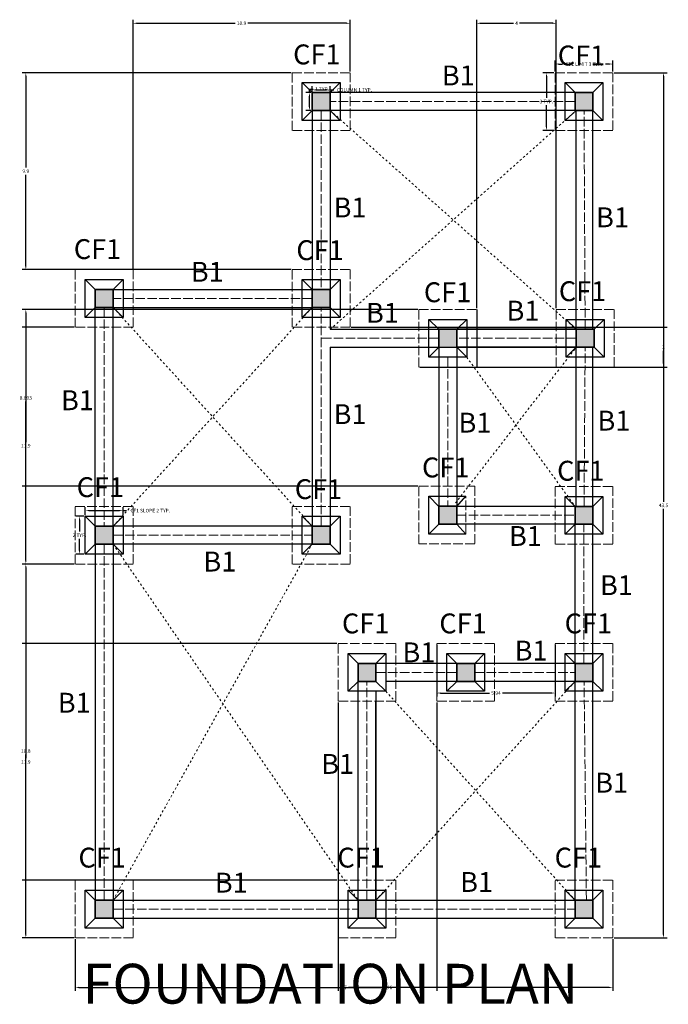
# Model space of a CAD drawing. Units: inches. Extents: x -193.8 to -127.9, y -122.4 to -72.3.
# Tile 2 of 2: x -160.4 to -127.9, y -121.8 to -72.3. Entities that reach past the tile are written whole.
import ezdxf

# ---------------------------------------------------------------- set-up
doc = ezdxf.new("R2010")
doc.units = ezdxf.units.IN
doc.header["$LTSCALE"] = 0.2
doc.header["$MEASUREMENT"] = 0
doc.linetypes.add('ACAD_ISO02W100', pattern=[15, 12, -3])
doc.linetypes.add('ACAD_ISO07W100', pattern=[3, 0, -3])
for name, color, linetype, lineweight in [('A-ANNO-DIMS', 2, 'Continuous', 18), ('S-ANNO-TEXT', 7, 'Continuous', 18), ('S-ANNO-TITL', 2, 'Continuous', 35), ('S-BEAM', 7, 'Continuous', 30), ('S-BEAM-CNTR', 8, 'ACAD_ISO02W100', 13), ('S-COLS', 7, 'Continuous', 35), ('S-COLS-PATT', 252, 'Continuous', 13), ('S-FNDN', 3, 'Continuous', 25), ('S-FNDN-DIAG', 8, 'ACAD_ISO07W100', 13), ('S-FNDN-HIDN', 3, 'ACAD_ISO02W100', 18)]:
    doc.layers.add(name, color=color, linetype=linetype, lineweight=lineweight)
doc.styles.get("Standard").update_dxf_attribs({"font": 'arial.ttf'})
doc.dimstyles.get("Standard").update_dxf_attribs({"dimtxt": 0.18, "dimasz": 0.18, "dimexe": 0.18, "dimexo": 0.0625, "dimgap": 0.09, "dimtad": 0, "dimtih": 1, "dimtoh": 1, "dimdec": 1, "dimzin": 0, "dimdsep": 46, "dimlunit": 4, "dimtxsty": 'Standard', "dimcen": 0.09, "dimadec": 0, "dimazin": 0, "dimtfac": 1, "dimtdec": 1, "dimtofl": 0, "dimtmove": 0, "dimatfit": 3, "dimfxl": 1, "dimtolj": 1, "dimtzin": 0, "dimarcsym": 0})

# ---------------------------------------------------------------- blocks, each defined once
blk = doc.blocks.new('FOOTING-CF1-SLOPED')
for p, q in [((0, 0), (0, 1.9)), ((0, 1.9), (1.9, 1.9)), ((1.9, 1.9), (1.9, 0)), ((1.9, 0), (0, 0))]:
    blk.add_line(p, q)
at = {"ltscale": 0.2}
for p, q in [((0, 1.9), (0.5, 1.4)), ((1.4, 1.4), (1.9, 1.9)), ((0, 0), (0.5, 0.5)), ((1.4, 0.5), (1.9, 0))]:
    blk.add_line(p, q, dxfattribs=at)
blk = doc.blocks.new('FOOTING-CF1-LIMIT')
at = {"ltscale": 0.2}
for p, q in [((0, 2.9), (2.9, 2.9)), ((0, 0), (0, 2.9)), ((2.9, 2.9), (2.9, 0)), ((2.9, 0), (0, 0))]:
    blk.add_line(p, q, dxfattribs=at)
blk = doc.blocks.new('COLUMN-SQUARE-PLAN')
for p, q in [((0, 0.9), (0.9, 0.9)), ((0, 0), (0, 0.9)), ((0.9, 0.9), (0.9, 0)), ((0.9, 0), (0, 0))]:
    blk.add_line(p, q)
blk = doc.blocks.new('*D19')
at = {"layer": 'A-ANNO-DIMS', "color": 0, "lineweight": -2, "ltscale": 0.2, "transparency": 16777216}
for p, q in [((-157.135, -97.158), (-157.135, -96.755)), ((-156.955, -96.935), (-155.415, -96.935)), ((-155.235, -97.158), (-155.235, -96.755)), ((-155.235, -96.935), (-155.055, -96.935))]:
    blk.add_line(p, q, dxfattribs=at)
at = {"layer": 'A-ANNO-DIMS', "color": 0, "ltscale": 0.2, "transparency": 16777216}
for points in [[(-156.955, -96.905), (-156.955, -96.965), (-157.135, -96.935)], [(-155.415, -96.905), (-155.415, -96.965), (-155.235, -96.935)]]:
    blk.add_solid(points, dxfattribs=at)
at = {"layer": 'Defpoints', "color": 0, "ltscale": 0.2, "transparency": 16777216}
for p in [(-155.235, -96.935), (-157.135, -97.22), (-155.235, -97.22)]:
    blk.add_point(p, dxfattribs=at)
at = {"layer": 'A-ANNO-DIMS', "color": 0, "ltscale": 0.2, "transparency": 16777216, "insert": (-153.871, -96.935), "char_height": 0.18, "attachment_point": 5}
blk.add_mtext('\\A1;CF1 SLOPE 2 TYP.', dxfattribs=at)
blk = doc.blocks.new('*D20')
at = {"layer": 'A-ANNO-DIMS', "color": 0, "lineweight": -2, "ltscale": 0.2, "transparency": 16777216}
for p, q in [((-157.198, -97.22), (-157.6, -97.22)), ((-157.42, -97.4), (-157.42, -97.99)), ((-157.42, -98.94), (-157.42, -98.35)), ((-157.198, -99.12), (-157.6, -99.12))]:
    blk.add_line(p, q, dxfattribs=at)
at = {"layer": 'A-ANNO-DIMS', "color": 0, "ltscale": 0.2, "transparency": 16777216}
for points in [[(-157.45, -97.4), (-157.39, -97.4), (-157.42, -97.22)], [(-157.45, -98.94), (-157.39, -98.94), (-157.42, -99.12)]]:
    blk.add_solid(points, dxfattribs=at)
at = {"layer": 'Defpoints', "color": 0, "ltscale": 0.2, "transparency": 16777216}
for p in [(-157.42, -97.22), (-157.135, -97.22), (-157.135, -99.12)]:
    blk.add_point(p, dxfattribs=at)
at = {"layer": 'A-ANNO-DIMS', "color": 0, "ltscale": 0.2, "transparency": 16777216, "insert": (-157.42, -98.17), "char_height": 0.18, "attachment_point": 5}
blk.add_mtext('\\A1;2 TYP.', dxfattribs=at)
blk = doc.blocks.new('*D21')
at = {"layer": 'A-ANNO-DIMS', "color": 0, "lineweight": -2, "ltscale": 0.2, "transparency": 16777216}
for p, q in [((-133.535, -74.858), (-133.535, -74.305)), ((-133.355, -74.485), (-133.171, -74.485)), ((-130.815, -74.485), (-130.999, -74.485)), ((-130.635, -74.858), (-130.635, -74.305))]:
    blk.add_line(p, q, dxfattribs=at)
at = {"layer": 'A-ANNO-DIMS', "color": 0, "ltscale": 0.2, "transparency": 16777216}
for points in [[(-133.355, -74.455), (-133.355, -74.515), (-133.535, -74.485)], [(-130.815, -74.455), (-130.815, -74.515), (-130.635, -74.485)]]:
    blk.add_solid(points, dxfattribs=at)
at = {"layer": 'Defpoints', "color": 0, "ltscale": 0.2, "transparency": 16777216}
for p in [(-133.535, -74.485), (-133.535, -74.92), (-130.635, -74.92)]:
    blk.add_point(p, dxfattribs=at)
at = {"layer": 'A-ANNO-DIMS', "color": 0, "ltscale": 0.2, "transparency": 16777216, "insert": (-132.085, -74.485), "char_height": 0.18, "attachment_point": 5}
blk.add_mtext('\\A1;CF1 LIMIT 3 TYP.', dxfattribs=at)
blk = doc.blocks.new('*D22')
at = {"layer": 'A-ANNO-DIMS', "color": 0, "lineweight": -2, "ltscale": 0.2, "transparency": 16777216}
for p, q in [((-133.598, -74.92), (-134.15, -74.92)), ((-133.97, -75.1), (-133.97, -76.188)), ((-133.97, -77.64), (-133.97, -76.552)), ((-133.598, -77.82), (-134.15, -77.82))]:
    blk.add_line(p, q, dxfattribs=at)
at = {"layer": 'A-ANNO-DIMS', "color": 0, "ltscale": 0.2, "transparency": 16777216}
for points in [[(-134, -75.1), (-133.94, -75.1), (-133.97, -74.92)], [(-134, -77.64), (-133.94, -77.64), (-133.97, -77.82)]]:
    blk.add_solid(points, dxfattribs=at)
at = {"layer": 'Defpoints', "color": 0, "ltscale": 0.2, "transparency": 16777216}
for p in [(-133.535, -74.92), (-133.97, -77.82), (-133.535, -77.82)]:
    blk.add_point(p, dxfattribs=at)
at = {"layer": 'A-ANNO-DIMS', "color": 0, "ltscale": 0.2, "transparency": 16777216, "insert": (-133.97, -76.37), "char_height": 0.18, "attachment_point": 5}
blk.add_mtext('\\A1;3 TYP.', dxfattribs=at)
blk = doc.blocks.new('*D23')
at = {"layer": 'A-ANNO-DIMS', "color": 0, "lineweight": -2, "ltscale": 0.2, "transparency": 16777216}
for p, q in [((-145.735, -75.858), (-145.735, -75.605)), ((-144.835, -75.858), (-144.835, -75.605)), ((-145.555, -75.785), (-145.015, -75.785)), ((-144.835, -75.785), (-144.655, -75.785))]:
    blk.add_line(p, q, dxfattribs=at)
at = {"layer": 'A-ANNO-DIMS', "color": 0, "ltscale": 0.2, "transparency": 16777216}
for points in [[(-145.555, -75.755), (-145.555, -75.815), (-145.735, -75.785)], [(-145.015, -75.755), (-145.015, -75.815), (-144.835, -75.785)]]:
    blk.add_solid(points, dxfattribs=at)
at = {"layer": 'Defpoints', "color": 0, "ltscale": 0.2, "transparency": 16777216}
for p in [(-145.735, -75.92), (-144.835, -75.785), (-144.835, -75.92)]:
    blk.add_point(p, dxfattribs=at)
at = {"layer": 'A-ANNO-DIMS', "color": 0, "ltscale": 0.2, "transparency": 16777216, "insert": (-143.618, -75.785), "char_height": 0.18, "attachment_point": 5}
blk.add_mtext('\\A1;COLUMN 1 TYP.', dxfattribs=at)
blk = doc.blocks.new('*D24')
at = {"layer": 'A-ANNO-DIMS', "color": 0, "lineweight": -2, "ltscale": 0.2, "transparency": 16777216}
for p, q in [((-145.798, -75.92), (-146.05, -75.92)), ((-145.87, -75.92), (-145.87, -75.74)), ((-145.87, -75.74), (-145.69, -75.74)), ((-145.87, -76.64), (-145.87, -76.1)), ((-145.798, -76.82), (-146.05, -76.82))]:
    blk.add_line(p, q, dxfattribs=at)
at = {"layer": 'A-ANNO-DIMS', "color": 0, "ltscale": 0.2, "transparency": 16777216}
for points in [[(-145.9, -76.1), (-145.84, -76.1), (-145.87, -75.92)], [(-145.9, -76.64), (-145.84, -76.64), (-145.87, -76.82)]]:
    blk.add_solid(points, dxfattribs=at)
at = {"layer": 'Defpoints', "color": 0, "ltscale": 0.2, "transparency": 16777216}
for p in [(-145.87, -75.92), (-145.735, -75.92), (-145.735, -76.82)]:
    blk.add_point(p, dxfattribs=at)
at = {"layer": 'A-ANNO-DIMS', "color": 0, "ltscale": 0.2, "transparency": 16777216, "insert": (-145.24, -75.74), "char_height": 0.18, "attachment_point": 5}
blk.add_mtext('\\A1;1 TYP.', dxfattribs=at)
blk = doc.blocks.new('*D44')
at = {"layer": 'A-ANNO-DIMS', "color": 0, "lineweight": -2, "ltscale": 0.2, "transparency": 16777216}
for p, q in [((-157.635, -118.483), (-157.635, -121.085)), ((-130.635, -118.483), (-130.635, -121.085)), ((-157.455, -120.905), (-144.356, -120.905)), ((-130.815, -120.905), (-143.915, -120.905))]:
    blk.add_line(p, q, dxfattribs=at)
at = {"layer": 'A-ANNO-DIMS', "color": 0, "ltscale": 0.2, "transparency": 16777216}
for points in [[(-157.455, -120.875), (-157.455, -120.935), (-157.635, -120.905)], [(-130.815, -120.875), (-130.815, -120.935), (-130.635, -120.905)]]:
    blk.add_solid(points, dxfattribs=at)
at = {"layer": 'Defpoints', "color": 0, "ltscale": 0.2, "transparency": 16777216}
for p in [(-157.635, -118.42), (-130.635, -118.42), (-130.635, -120.905)]:
    blk.add_point(p, dxfattribs=at)
at = {"layer": 'A-ANNO-DIMS', "color": 0, "ltscale": 0.2, "transparency": 16777216, "insert": (-144.135, -120.905), "char_height": 0.18, "attachment_point": 5}
blk.add_mtext('\\A1;27', dxfattribs=at)
blk = doc.blocks.new('*D45')
at = {"layer": 'A-ANNO-DIMS', "color": 0, "lineweight": -2, "ltscale": 0.2, "transparency": 16777216}
for p, q in [((-130.573, -74.92), (-127.91, -74.92)), ((-128.09, -75.1), (-128.09, -96.488)), ((-128.09, -118.24), (-128.09, -96.852)), ((-130.573, -118.42), (-127.91, -118.42))]:
    blk.add_line(p, q, dxfattribs=at)
at = {"layer": 'A-ANNO-DIMS', "color": 0, "ltscale": 0.2, "transparency": 16777216}
for points in [[(-128.12, -75.1), (-128.06, -75.1), (-128.09, -74.92)], [(-128.12, -118.24), (-128.06, -118.24), (-128.09, -118.42)]]:
    blk.add_solid(points, dxfattribs=at)
at = {"layer": 'Defpoints', "color": 0, "ltscale": 0.2, "transparency": 16777216}
for p in [(-130.635, -74.92), (-128.09, -74.92), (-130.635, -118.42)]:
    blk.add_point(p, dxfattribs=at)
at = {"layer": 'A-ANNO-DIMS', "color": 0, "ltscale": 0.2, "transparency": 16777216, "insert": (-128.09, -96.67), "char_height": 0.18, "attachment_point": 5}
blk.add_mtext('\\A1;43.5', dxfattribs=at)
blk = doc.blocks.new('*D46')
at = {"layer": 'A-ANNO-DIMS', "color": 0, "lineweight": -2, "ltscale": 0.2, "transparency": 16777216}
for p, q in [((-157.698, -99.62), (-160.3, -99.62)), ((-160.12, -99.8), (-160.12, -108.838)), ((-160.12, -118.24), (-160.12, -109.202)), ((-157.698, -118.42), (-160.3, -118.42))]:
    blk.add_line(p, q, dxfattribs=at)
at = {"layer": 'A-ANNO-DIMS', "color": 0, "ltscale": 0.2, "transparency": 16777216}
for points in [[(-160.15, -99.8), (-160.09, -99.8), (-160.12, -99.62)], [(-160.15, -118.24), (-160.09, -118.24), (-160.12, -118.42)]]:
    blk.add_solid(points, dxfattribs=at)
at = {"layer": 'Defpoints', "color": 0, "ltscale": 0.2, "transparency": 16777216}
for p in [(-157.635, -99.62), (-160.12, -118.42), (-157.635, -118.42)]:
    blk.add_point(p, dxfattribs=at)
at = {"layer": 'A-ANNO-DIMS', "color": 0, "ltscale": 0.2, "transparency": 16777216, "insert": (-160.12, -109.02), "char_height": 0.18, "attachment_point": 5}
blk.add_mtext('\\A1;18.8', dxfattribs=at)
blk = doc.blocks.new('*D47')
at = {"layer": 'A-ANNO-DIMS', "color": 0, "lineweight": -2, "ltscale": 0.2, "transparency": 16777216}
for p, q in [((-157.698, -87.72), (-160.3, -87.72)), ((-160.12, -87.9), (-160.12, -93.488)), ((-160.12, -99.44), (-160.12, -93.852)), ((-157.698, -99.62), (-160.3, -99.62))]:
    blk.add_line(p, q, dxfattribs=at)
at = {"layer": 'A-ANNO-DIMS', "color": 0, "ltscale": 0.2, "transparency": 16777216}
for points in [[(-160.15, -87.9), (-160.09, -87.9), (-160.12, -87.72)], [(-160.15, -99.44), (-160.09, -99.44), (-160.12, -99.62)]]:
    blk.add_solid(points, dxfattribs=at)
at = {"layer": 'Defpoints', "color": 0, "ltscale": 0.2, "transparency": 16777216}
for p in [(-157.635, -87.72), (-160.12, -99.62), (-157.635, -99.62)]:
    blk.add_point(p, dxfattribs=at)
at = {"layer": 'A-ANNO-DIMS', "color": 0, "ltscale": 0.2, "transparency": 16777216, "insert": (-160.12, -93.67), "char_height": 0.18, "attachment_point": 5}
blk.add_mtext('\\A1;11.9', dxfattribs=at)
blk = doc.blocks.new('*D48')
at = {"layer": 'A-ANNO-DIMS', "color": 0, "lineweight": -2, "ltscale": 0.2, "transparency": 16777216}
for p, q in [((-154.735, -84.758), (-154.735, -72.255)), ((-143.835, -74.858), (-143.835, -72.255)), ((-154.555, -72.435), (-149.601, -72.435)), ((-144.015, -72.435), (-148.97, -72.435))]:
    blk.add_line(p, q, dxfattribs=at)
at = {"layer": 'A-ANNO-DIMS', "color": 0, "ltscale": 0.2, "transparency": 16777216}
for points in [[(-154.555, -72.405), (-154.555, -72.465), (-154.735, -72.435)], [(-144.015, -72.405), (-144.015, -72.465), (-143.835, -72.435)]]:
    blk.add_solid(points, dxfattribs=at)
at = {"layer": 'Defpoints', "color": 0, "ltscale": 0.2, "transparency": 16777216}
for p in [(-143.835, -72.435), (-143.835, -74.92), (-154.735, -84.82)]:
    blk.add_point(p, dxfattribs=at)
at = {"layer": 'A-ANNO-DIMS', "color": 0, "ltscale": 0.2, "transparency": 16777216, "insert": (-149.285, -72.435), "char_height": 0.18, "attachment_point": 5}
blk.add_mtext('\\A1;10.9', dxfattribs=at)
blk = doc.blocks.new('*D49')
at = {"layer": 'A-ANNO-DIMS', "color": 0, "lineweight": -2, "ltscale": 0.2, "transparency": 16777216}
for p, q in [((-146.798, -74.92), (-160.3, -74.92)), ((-160.12, -75.1), (-160.12, -79.688)), ((-160.12, -84.64), (-160.12, -80.052)), ((-146.798, -84.82), (-160.3, -84.82))]:
    blk.add_line(p, q, dxfattribs=at)
at = {"layer": 'A-ANNO-DIMS', "color": 0, "ltscale": 0.2, "transparency": 16777216}
for points in [[(-160.15, -75.1), (-160.09, -75.1), (-160.12, -74.92)], [(-160.15, -84.64), (-160.09, -84.64), (-160.12, -84.82)]]:
    blk.add_solid(points, dxfattribs=at)
at = {"layer": 'Defpoints', "color": 0, "ltscale": 0.2, "transparency": 16777216}
for p in [(-160.12, -74.92), (-146.735, -74.92), (-146.735, -84.82)]:
    blk.add_point(p, dxfattribs=at)
at = {"layer": 'A-ANNO-DIMS', "color": 0, "ltscale": 0.2, "transparency": 16777216, "insert": (-160.12, -79.87), "char_height": 0.18, "attachment_point": 5}
blk.add_mtext('\\A1;9.9', dxfattribs=at)
blk = doc.blocks.new('*D50')
at = {"layer": 'A-ANNO-DIMS', "color": 0, "lineweight": -2, "ltscale": 0.2, "transparency": 16777216}
for p, q in [((-144.498, -103.62), (-160.3, -103.62)), ((-160.12, -103.8), (-160.12, -109.388)), ((-160.12, -115.34), (-160.12, -109.752)), ((-144.498, -115.52), (-160.3, -115.52))]:
    blk.add_line(p, q, dxfattribs=at)
at = {"layer": 'A-ANNO-DIMS', "color": 0, "ltscale": 0.2, "transparency": 16777216}
for points in [[(-160.15, -103.8), (-160.09, -103.8), (-160.12, -103.62)], [(-160.15, -115.34), (-160.09, -115.34), (-160.12, -115.52)]]:
    blk.add_solid(points, dxfattribs=at)
at = {"layer": 'Defpoints', "color": 0, "ltscale": 0.2, "transparency": 16777216}
for p in [(-160.12, -103.62), (-144.435, -103.62), (-144.435, -115.52)]:
    blk.add_point(p, dxfattribs=at)
at = {"layer": 'A-ANNO-DIMS', "color": 0, "ltscale": 0.2, "transparency": 16777216, "insert": (-160.12, -109.57), "char_height": 0.18, "attachment_point": 5}
blk.add_mtext('\\A1;11.9', dxfattribs=at)
blk = doc.blocks.new('*D51')
at = {"layer": 'A-ANNO-DIMS', "color": 0, "lineweight": -2, "ltscale": 0.2, "transparency": 16777216}
for p, q in [((-140.438, -86.82), (-160.3, -86.82)), ((-160.12, -87), (-160.12, -91.085)), ((-160.12, -95.533), (-160.12, -91.449)), ((-140.438, -95.713), (-160.3, -95.713))]:
    blk.add_line(p, q, dxfattribs=at)
at = {"layer": 'A-ANNO-DIMS', "color": 0, "ltscale": 0.2, "transparency": 16777216}
for points in [[(-160.15, -87), (-160.09, -87), (-160.12, -86.82)], [(-160.15, -95.533), (-160.09, -95.533), (-160.12, -95.713)]]:
    blk.add_solid(points, dxfattribs=at)
at = {"layer": 'Defpoints', "color": 0, "ltscale": 0.2, "transparency": 16777216}
for p in [(-140.375, -86.82), (-160.12, -95.713), (-140.375, -95.713)]:
    blk.add_point(p, dxfattribs=at)
at = {"layer": 'A-ANNO-DIMS', "color": 0, "ltscale": 0.2, "transparency": 16777216, "insert": (-160.12, -91.267), "char_height": 0.18, "attachment_point": 5}
blk.add_mtext('\\A1;8.893', dxfattribs=at)
blk = doc.blocks.new('*D52')
at = {"layer": 'A-ANNO-DIMS', "color": 0, "lineweight": -2, "ltscale": 0.2, "transparency": 16777216}
for p, q in [((-137.475, -86.758), (-137.475, -72.255)), ((-133.475, -86.758), (-133.475, -72.255)), ((-137.295, -72.435), (-135.627, -72.435)), ((-133.655, -72.435), (-135.323, -72.435))]:
    blk.add_line(p, q, dxfattribs=at)
at = {"layer": 'A-ANNO-DIMS', "color": 0, "ltscale": 0.2, "transparency": 16777216}
for points in [[(-137.295, -72.405), (-137.295, -72.465), (-137.475, -72.435)], [(-133.655, -72.405), (-133.655, -72.465), (-133.475, -72.435)]]:
    blk.add_solid(points, dxfattribs=at)
at = {"layer": 'Defpoints', "color": 0, "ltscale": 0.2, "transparency": 16777216}
for p in [(-133.475, -72.435), (-137.475, -86.82), (-133.475, -86.82)]:
    blk.add_point(p, dxfattribs=at)
at = {"layer": 'A-ANNO-DIMS', "color": 0, "ltscale": 0.2, "transparency": 16777216, "insert": (-135.475, -72.435), "char_height": 0.18, "attachment_point": 5}
blk.add_mtext('\\A1;4', dxfattribs=at)
blk = doc.blocks.new('*D53')
at = {"layer": 'A-ANNO-DIMS', "color": 0, "lineweight": -2, "ltscale": 0.2, "transparency": 16777216}
for p, q in [((-144.435, -106.583), (-144.435, -121.085)), ((-139.475, -106.583), (-139.475, -121.085)), ((-144.255, -120.905), (-142.282, -120.905)), ((-139.655, -120.905), (-141.628, -120.905))]:
    blk.add_line(p, q, dxfattribs=at)
at = {"layer": 'A-ANNO-DIMS', "color": 0, "ltscale": 0.2, "transparency": 16777216}
for points in [[(-144.255, -120.875), (-144.255, -120.935), (-144.435, -120.905)], [(-139.655, -120.875), (-139.655, -120.935), (-139.475, -120.905)]]:
    blk.add_solid(points, dxfattribs=at)
at = {"layer": 'Defpoints', "color": 0, "ltscale": 0.2, "transparency": 16777216}
for p in [(-144.435, -106.52), (-139.475, -106.52), (-139.475, -120.905)]:
    blk.add_point(p, dxfattribs=at)
at = {"layer": 'A-ANNO-DIMS', "color": 0, "ltscale": 0.2, "transparency": 16777216, "insert": (-141.955, -120.905), "char_height": 0.18, "attachment_point": 5}
blk.add_mtext('\\A1;4.96', dxfattribs=at)
blk = doc.blocks.new('*D54')
at = {"layer": 'A-ANNO-DIMS', "color": 0, "lineweight": -2, "ltscale": 0.2, "transparency": 16777216}
for p, q in [((-139.475, -103.683), (-139.475, -106.285)), ((-133.535, -103.683), (-133.535, -106.285)), ((-139.295, -106.105), (-136.828, -106.105)), ((-133.715, -106.105), (-136.182, -106.105))]:
    blk.add_line(p, q, dxfattribs=at)
at = {"layer": 'A-ANNO-DIMS', "color": 0, "ltscale": 0.2, "transparency": 16777216}
for points in [[(-139.295, -106.075), (-139.295, -106.135), (-139.475, -106.105)], [(-133.715, -106.075), (-133.715, -106.135), (-133.535, -106.105)]]:
    blk.add_solid(points, dxfattribs=at)
at = {"layer": 'Defpoints', "color": 0, "ltscale": 0.2, "transparency": 16777216}
for p in [(-139.475, -103.62), (-133.535, -103.62), (-139.475, -106.105)]:
    blk.add_point(p, dxfattribs=at)
at = {"layer": 'A-ANNO-DIMS', "color": 0, "ltscale": 0.2, "transparency": 16777216, "insert": (-136.505, -106.105), "char_height": 0.18, "attachment_point": 5}
blk.add_mtext('\\A1;5.94', dxfattribs=at)
blk = doc.blocks.new('*D55')
at = {"layer": 'A-ANNO-DIMS', "color": 0, "lineweight": -2, "ltscale": 0.2, "transparency": 16777216}
for p, q in [((-143.773, -87.72), (-127.91, -87.72)), ((-128.09, -87.9), (-128.09, -88.54)), ((-128.09, -89.54), (-128.09, -88.9)), ((-140.313, -89.72), (-127.91, -89.72))]:
    blk.add_line(p, q, dxfattribs=at)
at = {"layer": 'A-ANNO-DIMS', "color": 0, "ltscale": 0.2, "transparency": 16777216}
for points in [[(-128.12, -87.9), (-128.06, -87.9), (-128.09, -87.72)], [(-128.12, -89.54), (-128.06, -89.54), (-128.09, -89.72)]]:
    blk.add_solid(points, dxfattribs=at)
at = {"layer": 'Defpoints', "color": 0, "ltscale": 0.2, "transparency": 16777216}
for p in [(-143.835, -87.72), (-140.375, -89.72), (-128.09, -89.72)]:
    blk.add_point(p, dxfattribs=at)
at = {"layer": 'A-ANNO-DIMS', "color": 0, "ltscale": 0.2, "transparency": 16777216, "insert": (-128.09, -88.72), "char_height": 0.18, "attachment_point": 5}
blk.add_mtext('\\A1;2', dxfattribs=at)

msp = doc.modelspace()

# ---------------------------------------------------------------- hatches: boundary and pattern name
at = {"layer": 'S-COLS-PATT'}
h = msp.add_hatch(color=256, dxfattribs=at)
h.dxf.hatch_style = 1
h.paths.add_polyline_path([(-144.835, -75.9201), (-145.735, -75.9201), (-145.735, -76.8201), (-144.835, -76.8201)])
h.paths.add_polyline_path([(-131.635, -75.9201), (-132.535, -75.9201), (-132.535, -76.8201), (-131.635, -76.8201)])
h.paths.add_polyline_path([(-144.835, -85.8201), (-145.735, -85.8201), (-145.735, -86.7201), (-144.835, -86.7201)])
h.paths.add_polyline_path([(-155.735, -85.8201), (-156.635, -85.8201), (-156.635, -86.7201), (-155.735, -86.7201)])
h.paths.add_polyline_path([(-138.475, -87.8201), (-139.375, -87.8201), (-139.375, -88.7201), (-138.925, -88.7201), (-138.475, -88.7201)])
h.paths.add_polyline_path([(-131.575, -87.8201), (-132.475, -87.8201), (-132.475, -88.7201), (-131.575, -88.7201)])
h.paths.add_polyline_path([(-131.635, -96.7201), (-132.535, -96.7201), (-132.535, -97.6201), (-131.635, -97.6201)])
h.paths.add_polyline_path([(-138.475, -96.7201), (-138.475, -96.713), (-139.375, -96.713), (-139.375, -97.613), (-138.475, -97.613)])
h = msp.add_hatch(color=256, dxfattribs=at)
h.dxf.hatch_style = 1
h.paths.add_polyline_path([(-156.635, -97.7201), (-156.635, -98.6201), (-155.735, -98.6201), (-155.735, -97.7201)])
h.paths.add_polyline_path([(-144.835, -97.7201), (-145.735, -97.7201), (-145.735, -98.6201), (-144.835, -98.6201)])
h.paths.add_polyline_path([(-138.475, -104.6201), (-138.475, -105.5201), (-137.575, -105.5201), (-137.575, -104.6201)])
h.paths.add_polyline_path([(-132.535, -105.5201), (-131.635, -105.5201), (-131.635, -104.6201), (-132.535, -104.6201)])
h.paths.add_polyline_path([(-131.635, -116.5201), (-132.535, -116.5201), (-132.535, -117.4201), (-131.635, -117.4201)])
h.paths.add_polyline_path([(-142.535, -116.5201), (-143.435, -116.5201), (-143.435, -117.4201), (-142.535, -117.4201)])
h.paths.add_polyline_path([(-156.635, -116.5201), (-156.635, -117.4201), (-155.735, -117.4201), (-155.735, -116.5201)])
h = msp.add_hatch(color=256, dxfattribs=at)
h.dxf.hatch_style = 1
h.paths.add_polyline_path([(-143.435, -104.6201), (-143.435, -105.5201), (-142.535, -105.5201), (-142.535, -104.6201)])

# ---------------------------------------------------------------- linework, layer by layer
at = {"layer": 'S-BEAM'}
for p, q in [((-145.735, -75.9201), (-145.735, -85.8201)), ((-131.635, -75.9201), (-145.735, -75.9201)), ((-131.635, -87.8201), (-131.635, -75.9201)), ((-144.835, -76.8201), (-144.835, -87.8201)), ((-132.475, -76.8201), (-144.835, -76.8201)), ((-132.475, -87.8201), (-132.475, -76.8201)), ((-156.635, -85.8201), (-145.735, -85.8201)), ((-156.635, -98.6201), (-156.635, -85.8201)), ((-155.735, -86.7201), (-145.735, -86.7201)), ((-155.735, -97.7201), (-155.735, -86.7201)), ((-145.735, -86.7201), (-145.735, -93.6987)), ((-145.735, -86.7201), (-145.735, -97.7201)), ((-144.835, -87.8201), (-132.475, -87.8201)), ((-132.475, -87.8201), (-138.475, -87.8201)), ((-144.835, -88.7201), (-144.835, -97.7201)), ((-144.835, -88.7201), (-138.925, -88.7201)), ((-139.375, -88.7201), (-139.375, -96.7201)), ((-138.925, -88.7201), (-132.475, -88.7201)), ((-132.475, -88.7201), (-138.475, -88.7201)), ((-138.475, -88.7201), (-138.475, -96.7201)), ((-132.475, -96.7201), (-132.475, -88.7201)), ((-131.635, -104.6201), (-131.635, -88.7201)), ((-139.375, -96.713), (-139.375, -97.6201)), ((-132.475, -96.7201), (-138.475, -96.7201)), ((-156.635, -97.7201), (-156.635, -117.4201)), ((-145.735, -97.7201), (-155.735, -97.7201)), ((-144.835, -97.7201), (-144.835, -98.6201)), ((-138.475, -97.6201), (-139.375, -97.6201)), ((-138.475, -97.6201), (-139.375, -97.6201)), ((-132.535, -97.6201), (-138.475, -97.6201)), ((-132.535, -104.6201), (-132.535, -97.6201)), ((-144.835, -98.6201), (-155.735, -98.6201)), ((-155.735, -98.6201), (-155.735, -116.5201)), ((-143.435, -116.5201), (-143.435, -104.6201)), ((-138.475, -104.6201), (-143.435, -104.6201)), ((-132.535, -104.6201), (-137.575, -104.6201)), ((-131.635, -117.4201), (-131.635, -104.6201)), ((-132.535, -105.5201), (-142.035, -105.5201)), ((-132.535, -116.5201), (-132.535, -105.5201)), ((-142.535, -106.0201), (-142.535, -116.5201)), ((-142.535, -116.5201), (-142.535, -106.5201)), ((-155.735, -116.5201), (-143.435, -116.5201)), ((-142.535, -116.5201), (-132.535, -116.5201)), ((-156.635, -117.4201), (-143.435, -117.4201)), ((-143.435, -117.4201), (-131.635, -117.4201))]:
    msp.add_line(p, q, dxfattribs=at)
at = {"layer": 'S-BEAM-CNTR', "ltscale": 0.2}
for p, q in [((-132.535, -76.3701), (-144.835, -76.3701)), ((-145.285, -76.8201), (-145.285, -85.8201)), ((-132.0273, -87.8201), (-132.0828, -76.8201)), ((-145.735, -86.2701), (-155.735, -86.2701)), ((-156.185, -86.7201), (-156.185, -97.7201)), ((-145.285, -97.7201), (-145.285, -86.7201)), ((-139.375, -88.2701), (-145.285, -88.2701)), ((-132.475, -88.2701), (-138.475, -88.2701)), ((-132.082, -96.7201), (-132.0281, -88.7201)), ((-138.925, -89.2201), (-138.925, -96.7201)), ((-138.475, -97.1668), (-132.535, -97.1698)), ((-132.085, -104.6201), (-132.085, -97.613)), ((-155.735, -98.1701), (-145.735, -98.1701)), ((-156.185, -98.6201), (-156.185, -116.5201)), ((-142.535, -105.0701), (-138.475, -105.0701)), ((-137.575, -105.0701), (-132.535, -105.0701)), ((-142.985, -116.5201), (-142.985, -105.5201)), ((-131.9631, -116.5201), (-132.0803, -105.5201)), ((-155.735, -116.9701), (-143.435, -116.9701)), ((-142.535, -116.9701), (-132.535, -116.9701))]:
    msp.add_line(p, q, dxfattribs=at)
at = {"layer": 'S-COLS'}
for p, q in [((-139.375, -87.8201), (-138.475, -87.8201)), ((-139.375, -88.7201), (-139.375, -87.8201)), ((-138.475, -87.8201), (-138.475, -88.7201)), ((-139.375, -96.713), (-138.475, -96.713)), ((-139.375, -97.613), (-139.375, -96.713)), ((-138.475, -96.7201), (-138.475, -97.6201)), ((-156.635, -97.7201), (-155.735, -97.7201)), ((-156.635, -98.6201), (-156.635, -97.7201)), ((-155.735, -97.7201), (-155.735, -98.6201)), ((-145.735, -97.7201), (-144.835, -97.7201)), ((-145.735, -98.6201), (-145.735, -97.7201)), ((-144.835, -97.7201), (-144.835, -98.6201)), ((-138.475, -97.613), (-139.375, -97.613)), ((-155.735, -98.6201), (-156.635, -98.6201)), ((-144.835, -98.6201), (-145.735, -98.6201)), ((-143.435, -104.6201), (-142.535, -104.6201)), ((-143.435, -105.5201), (-143.435, -104.6201)), ((-142.535, -104.6201), (-142.535, -105.5201)), ((-138.475, -104.6201), (-137.575, -104.6201)), ((-138.475, -105.5201), (-138.475, -104.6201)), ((-137.575, -104.6201), (-137.575, -105.5201)), ((-132.535, -104.6201), (-131.635, -104.6201)), ((-132.535, -105.5201), (-132.535, -104.6201)), ((-131.635, -104.6201), (-131.635, -105.5201)), ((-142.535, -105.5201), (-143.435, -105.5201)), ((-137.575, -105.5201), (-138.475, -105.5201)), ((-131.635, -105.5201), (-132.535, -105.5201)), ((-156.635, -116.5201), (-155.735, -116.5201)), ((-156.635, -117.4201), (-156.635, -116.5201)), ((-155.735, -116.5201), (-155.735, -117.4201)), ((-143.435, -116.5201), (-142.535, -116.5201)), ((-143.435, -117.4201), (-143.435, -116.5201)), ((-142.535, -116.5201), (-142.535, -117.4201)), ((-132.535, -116.5201), (-131.635, -116.5201)), ((-132.535, -117.4201), (-132.535, -116.5201)), ((-131.635, -116.5201), (-131.635, -117.4201)), ((-155.735, -117.4201), (-156.635, -117.4201)), ((-142.535, -117.4201), (-143.435, -117.4201)), ((-131.635, -117.4201), (-132.535, -117.4201))]:
    msp.add_line(p, q, dxfattribs=at)
at = {"layer": 'S-FNDN'}
for p, q in [((-133.035, -75.4201), (-131.135, -75.4201)), ((-133.035, -77.3201), (-133.035, -75.4201)), ((-131.135, -75.4201), (-131.135, -77.3201)), ((-131.135, -77.3201), (-133.035, -77.3201)), ((-137.475, -86.8201), (-137.475, -89.7201)), ((-139.875, -98.113), (-139.875, -96.213)), ((-139.875, -96.213), (-138.025, -96.213)), ((-138.025, -98.113), (-139.875, -98.113))]:
    msp.add_line(p, q, dxfattribs=at)
at = {"layer": 'S-FNDN', "ltscale": 0.2}
for p, q in [((-132.535, -75.9201), (-133.035, -75.4201)), ((-131.635, -75.9201), (-131.135, -75.4201)), ((-132.475, -76.8201), (-133.035, -77.3201)), ((-131.635, -76.8201), (-131.135, -77.3201)), ((-139.375, -96.7201), (-139.875, -96.213)), ((-138.475, -96.7201), (-138.025, -96.213)), ((-139.375, -97.6201), (-139.875, -98.113)), ((-138.475, -97.6201), (-138.025, -98.113))]:
    msp.add_line(p, q, dxfattribs=at)
at = {"layer": 'S-FNDN-DIAG', "ltscale": 0.2}
for p, q in [((-144.835, -76.8201), (-132.475, -87.8201)), ((-144.835, -87.8201), (-132.475, -76.8201)), ((-155.735, -86.7201), (-145.735, -97.7201)), ((-155.735, -97.7201), (-145.735, -86.7201)), ((-138.535, -96.5497), (-132.475, -88.7201)), ((-137.975, -89.2201), (-132.535, -96.7201)), ((-155.735, -116.5201), (-145.735, -98.6201)), ((-155.735, -98.6201), (-143.435, -116.5201)), ((-142.535, -116.5201), (-132.535, -105.5201)), ((-142.035, -106.0201), (-132.535, -116.5201))]:
    msp.add_line(p, q, dxfattribs=at)
at = {"layer": 'S-FNDN-HIDN', "ltscale": 0.2}
for p, q in [((-140.375, -86.8201), (-137.475, -86.8201)), ((-140.375, -89.7201), (-140.375, -86.8201)), ((-137.475, -89.7201), (-140.375, -89.7201)), ((-140.375, -98.613), (-140.375, -95.713)), ((-140.375, -95.713), (-137.575, -95.713)), ((-137.575, -95.713), (-137.575, -98.613)), ((-138.025, -98.113), (-138.025, -96.213)), ((-137.575, -98.613), (-140.375, -98.613))]:
    msp.add_line(p, q, dxfattribs=at)

# ---------------------------------------------------------------- block references
at = {"layer": 'S-COLS'}
msp.add_blockref('COLUMN-SQUARE-PLAN', (-145.735, -76.8201), dxfattribs=at)
at = {"layer": 'S-COLS', "rotation": 180}
for p in [(-131.635, -75.9201), (-155.735, -85.8201), (-144.835, -85.8201), (-131.575, -87.8201), (-131.635, -96.7201)]:
    msp.add_blockref('COLUMN-SQUARE-PLAN', p, dxfattribs=at)
at = {"layer": 'S-FNDN'}
for p in [(-146.235, -77.3201), (-157.135, -87.2201), (-132.975, -89.2201), (-157.135, -99.1201), (-146.235, -99.1201), (-133.035, -106.0201), (-143.935, -117.9201)]:
    msp.add_blockref('FOOTING-CF1-SLOPED', p, dxfattribs=at)
for p, rotation in [((-146.235, -85.3201), 269.9999999999996), ((-139.875, -87.3201), 270), ((-131.135, -98.1201), 90), ((-142.035, -106.0201), 89.99999999999957), ((-137.075, -106.0201), 90.00000000000126), ((-155.235, -117.9201), 89.99999999999913), ((-133.035, -116.0201), 270.0000000000013)]:
    msp.add_blockref('FOOTING-CF1-SLOPED', p, dxfattribs=dict(at, rotation=rotation))
at = {"layer": 'S-FNDN-HIDN'}
for p, rotation in [((-146.735, -74.9201), 269.9999999999994), ((-130.635, -74.9201), 180), ((-146.735, -84.8201), 269.9999999999994), ((-133.475, -86.8201), 269.9999999999997), ((-143.835, -99.6201), 89.99999999999916), ((-141.535, -106.5201), 90.00000000000028), ((-133.535, -103.6201), 269.9999999999997), ((-154.735, -118.4201), 89.99999999999916)]:
    msp.add_blockref('FOOTING-CF1-LIMIT', p, dxfattribs=dict(at, rotation=rotation))
for p in [(-157.635, -87.7201), (-133.535, -98.6201), (-157.635, -99.6201), (-139.475, -106.5201), (-144.435, -118.4201), (-133.535, -118.4201)]:
    msp.add_blockref('FOOTING-CF1-LIMIT', p, dxfattribs=at)

# ---------------------------------------------------------------- texts
at = {"layer": 'S-ANNO-TEXT'}
for s, p in [('CF1', (-146.6946, -74.5013)), ('CF1', (-133.4013, -74.5542)), ('B1', (-139.224, -75.5581)), ('B1', (-144.6617, -82.1971)), ('B1', (-131.4793, -82.6909)), ('CF1', (-157.7106, -84.2887)), ('CF1', (-146.5357, -84.3416)), ('B1', (-151.8348, -85.4294)), ('CF1', (-140.1274, -86.4578)), ('CF1', (-133.3483, -86.4049)), ('B1', (-143.0359, -87.4911)), ('B1', (-135.975, -87.3826)), ('B1', (-158.3525, -91.8859)), ('B1', (-144.6607, -92.5864)), ('B1', (-138.387, -93.013)), ('B1', (-131.408, -92.9119)), ('CF1', (-140.2218, -95.2649)), ('CF1', (-133.4355, -95.4303)), ('CF1', (-157.5683, -96.257)), ('CF1', (-146.6109, -96.3562)), ('B1', (-135.8518, -98.7097)), ('B1', (-151.2005, -99.9968)), ('B1', (-131.2816, -101.1837)), ('CF1', (-144.242, -103.107)), ('CF1', (-139.3517, -103.107)), ('CF1', (-133.0583, -103.107)), ('B1', (-141.203, -104.5603)), ('B1', (-135.569, -104.4723)), ('B1', (-158.5152, -107.0946)), ('B1', (-145.2826, -110.1699)), ('B1', (-131.5211, -111.1133)), ('CF1', (-157.4769, -114.8792)), ('CF1', (-144.4725, -114.8792)), ('CF1', (-133.5603, -114.8792)), ('B1', (-150.6291, -116.1381)), ('B1', (-138.3068, -116.1044))]:
    msp.add_text(s, height=1, dxfattribs=at).set_placement(p)
at = {"layer": 'S-ANNO-TITL', "ltscale": 0.2}
msp.add_text('FOUNDATION PLAN', height=2, dxfattribs=at).set_placement((-157.2731, -121.7187))

# ---------------------------------------------------------------- dimensions: what is measured, and where the dimension line sits
at = {"layer": 'A-ANNO-DIMS', "ltscale": 0.2}
for base, p1, p2, override, picture, middle in [((-143.835, -72.4351), (-154.735, -84.8201), (-143.835, -74.9201), {"dimdec": 1, "dimlfac": 1, "dimrnd": 0, "dimzin": 0, "dimdsep": 46, "dimlunit": 2}, '*D48', (-149.285, -72.4351)), ((-133.475, -72.4351), (-137.475, -86.8201), (-133.475, -86.8201), {"dimdec": 0, "dimlfac": 1, "dimrnd": 0, "dimzin": 0, "dimdsep": 46, "dimlunit": 2}, '*D52', (-135.475, -72.4351)), ((-139.475, -120.9051), (-144.435, -106.5201), (-139.475, -106.5201), {"dimdec": 2, "dimlfac": 1, "dimrnd": 0, "dimzin": 0, "dimdsep": 46, "dimlunit": 2}, '*D53', (-141.955, -120.9051)), ((-130.635, -120.9051), (-157.635, -118.4201), (-130.635, -118.4201), {"dimdec": 0, "dimlfac": 1, "dimrnd": 0, "dimzin": 0, "dimdsep": 46, "dimlunit": 2}, '*D44', (-144.135, -120.9051))]:
    dim = msp.add_linear_dim(base=base, p1=p1, p2=p2, dimstyle='Standard', override=override, dxfattribs=at)
    dim.commit()
    dim.dimension.update_dxf_attribs({"geometry": picture, "text_midpoint": middle})
for base, p1, p2, angle, text, picture, middle in [((-133.535, -74.4851), (-130.635, -74.9201), (-133.535, -74.9201), 180, 'CF1 LIMIT <> TYP.', '*D21', (-132.085, -74.4851)), ((-133.97, -77.8201), (-133.535, -74.9201), (-133.535, -77.8201), 270, '<> TYP.', '*D22', (-133.97, -76.3701)), ((-145.87, -75.9201), (-145.735, -76.8201), (-145.735, -75.9201), 90, '<> TYP.', '*D24', (-145.2404, -75.7401)), ((-157.42, -97.2201), (-157.135, -99.1201), (-157.135, -97.2201), 90, '<> TYP.', '*D20', (-157.42, -98.1701))]:
    dim = msp.add_linear_dim(base=base, p1=p1, p2=p2, angle=angle, text=text, dimstyle='Standard', override={"dimdec": 0, "dimlfac": 1, "dimrnd": 0, "dimzin": 0, "dimdsep": 46, "dimlunit": 2}, dxfattribs=at)
    dim.commit()
    dim.dimension.update_dxf_attribs({"geometry": picture, "text_midpoint": middle})
for base, p1, p2, angle, override, picture, middle in [((-160.12, -74.9201), (-146.735, -84.8201), (-146.735, -74.9201), 90, {"dimdec": 1, "dimlfac": 1, "dimrnd": 0, "dimzin": 0, "dimdsep": 46, "dimlunit": 2}, '*D49', (-160.12, -79.8701)), ((-128.09, -74.9201), (-130.635, -118.4201), (-130.635, -74.9201), 90, {"dimdec": 1, "dimlfac": 1, "dimrnd": 0, "dimzin": 0, "dimdsep": 46, "dimlunit": 2}, '*D45', (-128.09, -96.6701)), ((-160.12, -95.713), (-140.375, -86.8201), (-140.375, -95.713), 90, {"dimdec": 3, "dimlfac": 1, "dimrnd": 0, "dimzin": 0, "dimdsep": 46, "dimlunit": 2}, '*D51', (-160.12, -91.2665)), ((-160.12, -99.6201), (-157.635, -87.7201), (-157.635, -99.6201), 90, {"dimdec": 1, "dimlfac": 1, "dimrnd": 0, "dimzin": 0, "dimdsep": 46, "dimlunit": 2}, '*D47', (-160.12, -93.6701)), ((-128.09, -89.7201), (-143.835, -87.7201), (-140.375, -89.7201), 90, {"dimdec": 0, "dimlfac": 1, "dimrnd": 0, "dimzin": 0, "dimdsep": 46, "dimlunit": 2}, '*D55', (-128.09, -88.7201)), ((-160.12, -118.4201), (-157.635, -99.6201), (-157.635, -118.4201), 90, {"dimdec": 1, "dimlfac": 1, "dimrnd": 0, "dimzin": 0, "dimdsep": 46, "dimlunit": 2}, '*D46', (-160.12, -109.0201)), ((-160.12, -103.6201), (-144.435, -115.5201), (-144.435, -103.6201), 90, {"dimdec": 1, "dimlfac": 1, "dimrnd": 0, "dimzin": 0, "dimdsep": 46, "dimlunit": 2}, '*D50', (-160.12, -109.5701)), ((-139.475, -106.1051), (-133.535, -103.6201), (-139.475, -103.6201), 180, {"dimdec": 2, "dimlfac": 1, "dimrnd": 0, "dimzin": 0, "dimdsep": 46, "dimlunit": 2}, '*D54', (-136.505, -106.1051))]:
    dim = msp.add_linear_dim(base=base, p1=p1, p2=p2, angle=angle, dimstyle='Standard', override=override, dxfattribs=at)
    dim.commit()
    dim.dimension.update_dxf_attribs({"geometry": picture, "text_midpoint": middle})
for base, p1, p2, text, picture, middle in [((-144.835, -75.7851), (-145.735, -75.9201), (-144.835, -75.9201), 'COLUMN <> TYP.', '*D23', (-143.6181, -75.7851)), ((-155.235, -96.9351), (-157.135, -97.2201), (-155.235, -97.2201), 'CF1 SLOPE <> TYP.', '*D19', (-153.8712, -96.9351))]:
    dim = msp.add_linear_dim(base=base, p1=p1, p2=p2, text=text, dimstyle='Standard', override={"dimdec": 0, "dimlfac": 1, "dimrnd": 0, "dimzin": 0, "dimdsep": 46, "dimlunit": 2}, dxfattribs=at)
    dim.commit()
    dim.dimension.update_dxf_attribs({"geometry": picture, "text_midpoint": middle})

doc.saveas('drawing.dxf')
